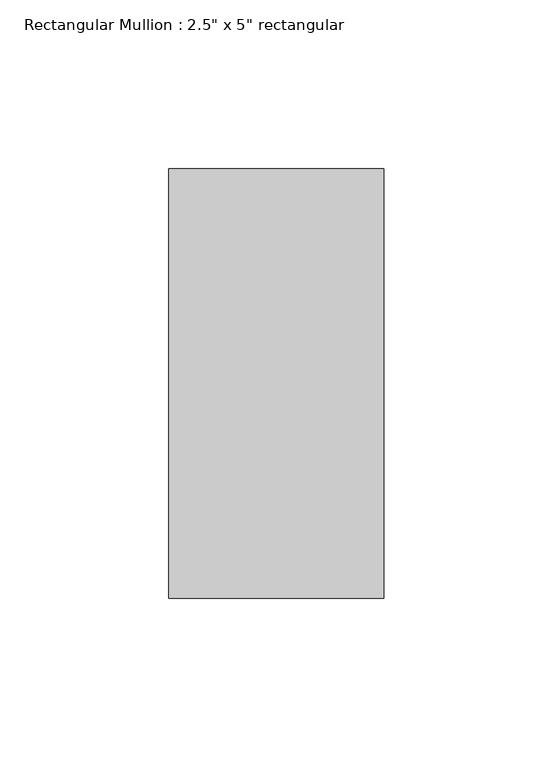
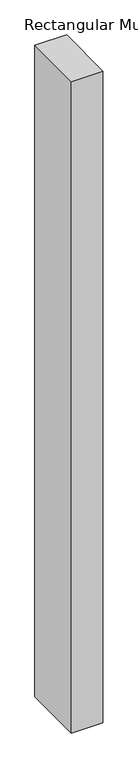
"""IFC4 building model written with IfcOpenShell, lengths in millimetres: member geometry."""

from ifc_helpers import new_model, si_unit, frame, origin, place, context, project, spatial, polyline, outline, extrude, source, transform, mapped, element, save


def member_e1cf819f(model_context):
    return source(origin(), model_context, "Body", "SweptSolid", [
        extrude(outline(polyline([(0.0, 63.5), (0.0, -63.5), (-63.5, -63.5), (-63.5, 63.5), (0.0, 63.5)])), frame((0.0, 0.0, -1384.3), z_axis=(0.0, 0.0, 1.0), x_axis=(1.0, 0.0, 0.0)), (0.0, 0.0, 1.0), 1384.3),
    ])


if __name__ == "__main__":
    model = new_model("IFC4")
    model_context = context("Model", 3, world=origin())
    ifc_project = project(units=[si_unit("LENGTHUNIT", "METRE", prefix="MILLI")], contexts=[model_context])
    site = spatial("IfcSite", under=ifc_project)
    building = spatial("IfcBuilding", under=site)
    placement = place(None, origin())
    member_shape = member_e1cf819f(model_context)
    element("IfcMember", 1, ObjectType="Rectangular Mullion : 2.5\" x 5\" rectangular", at=placement, inside=building, context=model_context, shape_type="MappedRepresentation", body=[
        mapped(member_shape, transform((0.0, 0.0, 0.0), x_axis=(1.0, 0.0, 0.0), y_axis=(0.0, 1.0, 0.0), z_axis=(0.0, 0.0, 1.0))),
    ])
    save(model, "model.ifc")

# Revit data of these elements
# Type "Rectangular Mullion : 2.5\" x 5\" rectangular"
#   built-in parameter 1007304 = 0.416667 (stored number, unit not read)
#   built-in parameter 1007301 = 0.104167 (stored number, unit not read)
#   built-in parameter 1007300 = 0.104167 (stored number, unit not read)
# Element 1 (IfcMember, "Rectangular Mullion : 2.5\" x 5\" rectangular")
#   Materials on its faces: "Aluminum"
# Materials
#   "Aluminum": class "Metal", colour RGB 247 247 247, transparency 0, Description = "Aluminum 6061", Cost = 0
